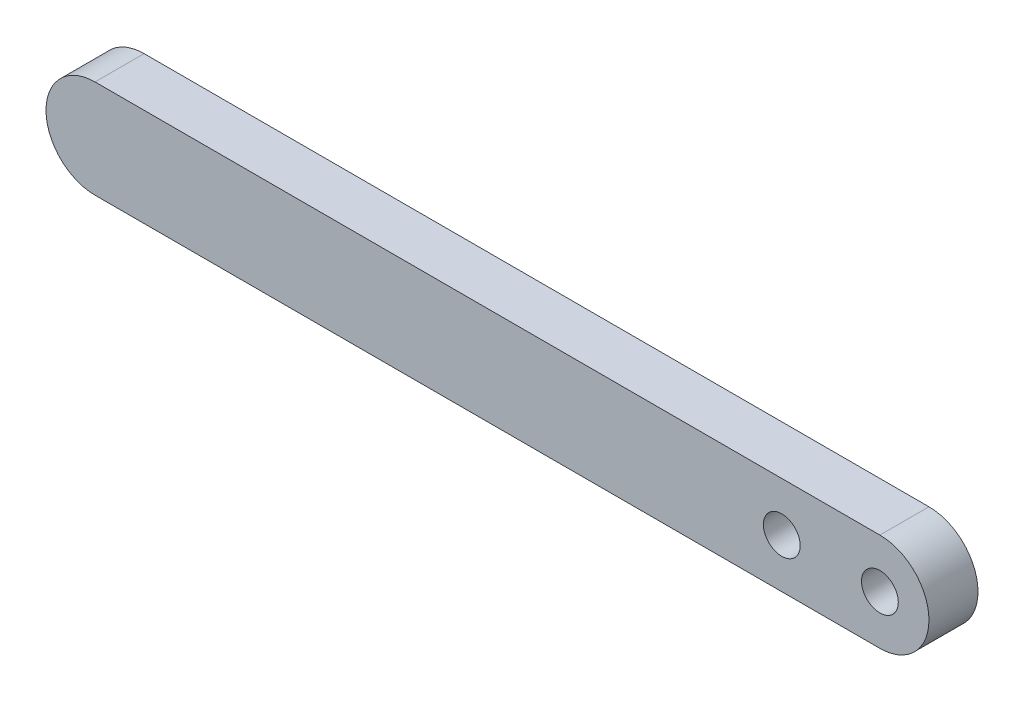
ISO-10303-21;
HEADER;
FILE_DESCRIPTION(('STEP AP214'),'2;1');
FILE_NAME('part.step','',(''),(''),'','','');
FILE_SCHEMA(('AUTOMOTIVE_DESIGN { 1 0 10303 214 1 1 1 1 }'));
ENDSEC;
DATA;
#1=APPLICATION_CONTEXT('core data for automotive mechanical design processes');
#2=APPLICATION_PROTOCOL_DEFINITION('international standard','automotive_design',2000,#1);
#3=PRODUCT_CONTEXT('',#1,'mechanical');
#4=PRODUCT('Part','Part','',(#3));
#5=PRODUCT_RELATED_PRODUCT_CATEGORY('part','',(#4));
#6=PRODUCT_DEFINITION_FORMATION('','',#4);
#7=PRODUCT_DEFINITION_CONTEXT('part definition',#1,'design');
#8=PRODUCT_DEFINITION('design','',#6,#7);
#9=PRODUCT_DEFINITION_SHAPE('','',#8);
#10=(LENGTH_UNIT() NAMED_UNIT(*) SI_UNIT(.MILLI.,.METRE.));
#11=(NAMED_UNIT(*) PLANE_ANGLE_UNIT() SI_UNIT($,.RADIAN.));
#12=(NAMED_UNIT(*) SI_UNIT($,.STERADIAN.) SOLID_ANGLE_UNIT());
#13=UNCERTAINTY_MEASURE_WITH_UNIT(LENGTH_MEASURE(1.E-05),#10,'distance_accuracy_value','');
#14=(GEOMETRIC_REPRESENTATION_CONTEXT(3) GLOBAL_UNCERTAINTY_ASSIGNED_CONTEXT((#13)) GLOBAL_UNIT_ASSIGNED_CONTEXT((#10,
#11,#12)) REPRESENTATION_CONTEXT('',''));
#15=CARTESIAN_POINT('',(0.,0.,0.));
#16=DIRECTION('',(0.,0.,1.));
#17=DIRECTION('',(1.,0.,0.));
#18=AXIS2_PLACEMENT_3D('',#15,#16,#17);
#19=CARTESIAN_POINT('',(-50.8,0.,3.175));
#20=DIRECTION('',(0.,0.,1.));
#21=DIRECTION('',(1.,0.,0.));
#22=AXIS2_PLACEMENT_3D('',#19,#20,#21);
#23=PLANE('',#22);
#24=CARTESIAN_POINT('',(50.8,0.,3.175));
#25=DIRECTION('',(0.,0.,1.));
#26=DIRECTION('',(1.,0.,0.));
#27=AXIS2_PLACEMENT_3D('',#24,#25,#26);
#28=CIRCLE('',#27,2.38125000000001);
#29=CARTESIAN_POINT('',(53.18125,0.,3.175));
#30=VERTEX_POINT('',#29);
#31=EDGE_CURVE('E106',#30,#30,#28,.T.);
#32=ORIENTED_EDGE('',*,*,#31,.F.);
#33=EDGE_LOOP('',(#32));
#34=FACE_BOUND('',#33,.T.);
#35=CARTESIAN_POINT('',(-50.8,0.,3.175));
#36=DIRECTION('',(0.,0.,1.));
#37=DIRECTION('',(1.,0.,0.));
#38=AXIS2_PLACEMENT_3D('',#35,#36,#37);
#39=CIRCLE('',#38,6.35000000000002);
#40=CARTESIAN_POINT('',(-50.8,6.35000000000002,3.175));
#41=VERTEX_POINT('',#40);
#42=CARTESIAN_POINT('',(-50.8,-6.35000000000002,3.175));
#43=VERTEX_POINT('',#42);
#44=EDGE_CURVE('E93',#41,#43,#39,.T.);
#45=ORIENTED_EDGE('',*,*,#44,.T.);
#46=DIRECTION('',(1.,0.,0.));
#47=VECTOR('',#46,1.);
#48=CARTESIAN_POINT('',(-50.8,-6.35000000000002,3.175));
#49=LINE('',#48,#47);
#50=CARTESIAN_POINT('',(50.8,-6.35000000000002,3.175));
#51=VERTEX_POINT('',#50);
#52=EDGE_CURVE('E88',#43,#51,#49,.T.);
#53=ORIENTED_EDGE('',*,*,#52,.T.);
#54=CARTESIAN_POINT('',(50.8,0.,3.175));
#55=DIRECTION('',(0.,0.,1.));
#56=DIRECTION('',(1.,0.,0.));
#57=AXIS2_PLACEMENT_3D('',#54,#55,#56);
#58=CIRCLE('',#57,6.35000000000002);
#59=CARTESIAN_POINT('',(50.8,6.35000000000004,3.175));
#60=VERTEX_POINT('',#59);
#61=EDGE_CURVE('E90',#51,#60,#58,.T.);
#62=ORIENTED_EDGE('',*,*,#61,.T.);
#63=DIRECTION('',(-1.,0.,0.));
#64=VECTOR('',#63,1.);
#65=CARTESIAN_POINT('',(-50.8,6.35000000000002,3.175));
#66=LINE('',#65,#64);
#67=EDGE_CURVE('E57',#60,#41,#66,.T.);
#68=ORIENTED_EDGE('',*,*,#67,.T.);
#69=EDGE_LOOP('',(#45,#53,#62,#68));
#70=FACE_BOUND('',#69,.T.);
#71=CARTESIAN_POINT('',(38.1,0.,3.175));
#72=DIRECTION('',(0.,0.,1.));
#73=DIRECTION('',(1.,0.,0.));
#74=AXIS2_PLACEMENT_3D('',#71,#72,#73);
#75=CIRCLE('',#74,2.38125);
#76=CARTESIAN_POINT('',(40.48125,0.,3.175));
#77=VERTEX_POINT('',#76);
#78=EDGE_CURVE('E122',#77,#77,#75,.T.);
#79=ORIENTED_EDGE('',*,*,#78,.F.);
#80=EDGE_LOOP('',(#79));
#81=FACE_BOUND('',#80,.T.);
#82=ADVANCED_FACE('F39',(#34,#70,#81),#23,.T.);
#83=CARTESIAN_POINT('',(-50.8,0.,-3.175));
#84=DIRECTION('',(0.,0.,1.));
#85=DIRECTION('',(1.,0.,0.));
#86=AXIS2_PLACEMENT_3D('',#83,#84,#85);
#87=PLANE('',#86);
#88=CARTESIAN_POINT('',(-50.8,0.,-3.175));
#89=DIRECTION('',(0.,0.,1.));
#90=DIRECTION('',(1.,0.,0.));
#91=AXIS2_PLACEMENT_3D('',#88,#89,#90);
#92=CIRCLE('',#91,6.35000000000002);
#93=CARTESIAN_POINT('',(-50.8,6.35000000000002,-3.175));
#94=VERTEX_POINT('',#93);
#95=CARTESIAN_POINT('',(-50.8,-6.35000000000002,-3.175));
#96=VERTEX_POINT('',#95);
#97=EDGE_CURVE('E103',#94,#96,#92,.T.);
#98=ORIENTED_EDGE('',*,*,#97,.F.);
#99=DIRECTION('',(-1.,0.,0.));
#100=VECTOR('',#99,1.);
#101=CARTESIAN_POINT('',(-50.8,6.35000000000002,-3.175));
#102=LINE('',#101,#100);
#103=CARTESIAN_POINT('',(50.8,6.35000000000004,-3.175));
#104=VERTEX_POINT('',#103);
#105=EDGE_CURVE('E76',#104,#94,#102,.T.);
#106=ORIENTED_EDGE('',*,*,#105,.F.);
#107=CARTESIAN_POINT('',(50.8,0.,-3.175));
#108=DIRECTION('',(0.,0.,1.));
#109=DIRECTION('',(1.,0.,0.));
#110=AXIS2_PLACEMENT_3D('',#107,#108,#109);
#111=CIRCLE('',#110,6.35000000000002);
#112=CARTESIAN_POINT('',(50.8,-6.35000000000002,-3.175));
#113=VERTEX_POINT('',#112);
#114=EDGE_CURVE('E71',#113,#104,#111,.T.);
#115=ORIENTED_EDGE('',*,*,#114,.F.);
#116=DIRECTION('',(1.,0.,0.));
#117=VECTOR('',#116,1.);
#118=CARTESIAN_POINT('',(-50.8,-6.35000000000002,-3.175));
#119=LINE('',#118,#117);
#120=EDGE_CURVE('E92',#96,#113,#119,.T.);
#121=ORIENTED_EDGE('',*,*,#120,.F.);
#122=EDGE_LOOP('',(#98,#106,#115,#121));
#123=FACE_BOUND('',#122,.T.);
#124=CARTESIAN_POINT('',(50.8,0.,-3.175));
#125=DIRECTION('',(0.,0.,1.));
#126=DIRECTION('',(1.,0.,0.));
#127=AXIS2_PLACEMENT_3D('',#124,#125,#126);
#128=CIRCLE('',#127,2.38125000000001);
#129=CARTESIAN_POINT('',(53.18125,0.,-3.175));
#130=VERTEX_POINT('',#129);
#131=EDGE_CURVE('E119',#130,#130,#128,.T.);
#132=ORIENTED_EDGE('',*,*,#131,.T.);
#133=EDGE_LOOP('',(#132));
#134=FACE_BOUND('',#133,.T.);
#135=CARTESIAN_POINT('',(38.1,0.,-3.175));
#136=DIRECTION('',(0.,0.,1.));
#137=DIRECTION('',(1.,0.,0.));
#138=AXIS2_PLACEMENT_3D('',#135,#136,#137);
#139=CIRCLE('',#138,2.38125);
#140=CARTESIAN_POINT('',(40.48125,0.,-3.175));
#141=VERTEX_POINT('',#140);
#142=EDGE_CURVE('E121',#141,#141,#139,.T.);
#143=ORIENTED_EDGE('',*,*,#142,.T.);
#144=EDGE_LOOP('',(#143));
#145=FACE_BOUND('',#144,.T.);
#146=ADVANCED_FACE('F111',(#123,#134,#145),#87,.F.);
#147=CARTESIAN_POINT('',(-50.8,0.,3.175));
#148=DIRECTION('',(0.,0.,-1.));
#149=DIRECTION('',(-1.,0.,0.));
#150=AXIS2_PLACEMENT_3D('',#147,#148,#149);
#151=CYLINDRICAL_SURFACE('',#150,6.35000000000002);
#152=ORIENTED_EDGE('',*,*,#97,.T.);
#153=DIRECTION('',(0.,0.,-1.));
#154=VECTOR('',#153,1.);
#155=CARTESIAN_POINT('',(-50.8,-6.35000000000002,3.175));
#156=LINE('',#155,#154);
#157=EDGE_CURVE('E11',#43,#96,#156,.T.);
#158=ORIENTED_EDGE('',*,*,#157,.F.);
#159=ORIENTED_EDGE('',*,*,#44,.F.);
#160=DIRECTION('',(0.,0.,-1.));
#161=VECTOR('',#160,1.);
#162=CARTESIAN_POINT('',(-50.8,6.35000000000002,3.175));
#163=LINE('',#162,#161);
#164=EDGE_CURVE('E97',#41,#94,#163,.T.);
#165=ORIENTED_EDGE('',*,*,#164,.T.);
#166=EDGE_LOOP('',(#152,#158,#159,#165));
#167=FACE_BOUND('',#166,.T.);
#168=ADVANCED_FACE('F41',(#167),#151,.T.);
#169=CARTESIAN_POINT('',(-50.8,-6.35000000000002,3.175));
#170=DIRECTION('',(0.,1.,0.));
#171=DIRECTION('',(-1.,0.,0.));
#172=AXIS2_PLACEMENT_3D('',#169,#170,#171);
#173=PLANE('',#172);
#174=ORIENTED_EDGE('',*,*,#120,.T.);
#175=DIRECTION('',(0.,0.,-1.));
#176=VECTOR('',#175,1.);
#177=CARTESIAN_POINT('',(50.8,-6.35000000000002,3.175));
#178=LINE('',#177,#176);
#179=EDGE_CURVE('E48',#51,#113,#178,.T.);
#180=ORIENTED_EDGE('',*,*,#179,.F.);
#181=ORIENTED_EDGE('',*,*,#52,.F.);
#182=ORIENTED_EDGE('',*,*,#157,.T.);
#183=EDGE_LOOP('',(#174,#180,#181,#182));
#184=FACE_BOUND('',#183,.T.);
#185=ADVANCED_FACE('F94',(#184),#173,.F.);
#186=CARTESIAN_POINT('',(50.8,0.,3.175));
#187=DIRECTION('',(0.,0.,-1.));
#188=DIRECTION('',(-1.,0.,0.));
#189=AXIS2_PLACEMENT_3D('',#186,#187,#188);
#190=CYLINDRICAL_SURFACE('',#189,6.35000000000002);
#191=ORIENTED_EDGE('',*,*,#114,.T.);
#192=DIRECTION('',(0.,0.,-1.));
#193=VECTOR('',#192,1.);
#194=CARTESIAN_POINT('',(50.8,6.35000000000004,3.175));
#195=LINE('',#194,#193);
#196=EDGE_CURVE('E96',#60,#104,#195,.T.);
#197=ORIENTED_EDGE('',*,*,#196,.F.);
#198=ORIENTED_EDGE('',*,*,#61,.F.);
#199=ORIENTED_EDGE('',*,*,#179,.T.);
#200=EDGE_LOOP('',(#191,#197,#198,#199));
#201=FACE_BOUND('',#200,.T.);
#202=ADVANCED_FACE('F100',(#201),#190,.T.);
#203=CARTESIAN_POINT('',(-50.8,6.35000000000002,3.175));
#204=DIRECTION('',(0.,-1.,0.));
#205=DIRECTION('',(1.,0.,0.));
#206=AXIS2_PLACEMENT_3D('',#203,#204,#205);
#207=PLANE('',#206);
#208=ORIENTED_EDGE('',*,*,#105,.T.);
#209=ORIENTED_EDGE('',*,*,#164,.F.);
#210=ORIENTED_EDGE('',*,*,#67,.F.);
#211=ORIENTED_EDGE('',*,*,#196,.T.);
#212=EDGE_LOOP('',(#208,#209,#210,#211));
#213=FACE_BOUND('',#212,.T.);
#214=ADVANCED_FACE('F112',(#213),#207,.F.);
#215=CARTESIAN_POINT('',(50.8,0.,3.175));
#216=DIRECTION('',(0.,0.,-1.));
#217=DIRECTION('',(-1.,0.,0.));
#218=AXIS2_PLACEMENT_3D('',#215,#216,#217);
#219=CYLINDRICAL_SURFACE('',#218,2.38125000000001);
#220=ORIENTED_EDGE('',*,*,#31,.T.);
#221=EDGE_LOOP('',(#220));
#222=FACE_BOUND('',#221,.T.);
#223=ORIENTED_EDGE('',*,*,#131,.F.);
#224=EDGE_LOOP('',(#223));
#225=FACE_BOUND('',#224,.T.);
#226=ADVANCED_FACE('F143',(#222,#225),#219,.F.);
#227=CARTESIAN_POINT('',(38.1,0.,3.175));
#228=DIRECTION('',(0.,0.,-1.));
#229=DIRECTION('',(-1.,0.,0.));
#230=AXIS2_PLACEMENT_3D('',#227,#228,#229);
#231=CYLINDRICAL_SURFACE('',#230,2.38125);
#232=ORIENTED_EDGE('',*,*,#78,.T.);
#233=EDGE_LOOP('',(#232));
#234=FACE_BOUND('',#233,.T.);
#235=ORIENTED_EDGE('',*,*,#142,.F.);
#236=EDGE_LOOP('',(#235));
#237=FACE_BOUND('',#236,.T.);
#238=ADVANCED_FACE('F128',(#234,#237),#231,.F.);
#239=CLOSED_SHELL('',(#82,#146,#168,#185,#202,#214,#226,#238));
#240=MANIFOLD_SOLID_BREP('B2',#239);
#241=ADVANCED_BREP_SHAPE_REPRESENTATION('',(#18,#240),#14);
#242=SHAPE_DEFINITION_REPRESENTATION(#9,#241);
ENDSEC;
END-ISO-10303-21;
